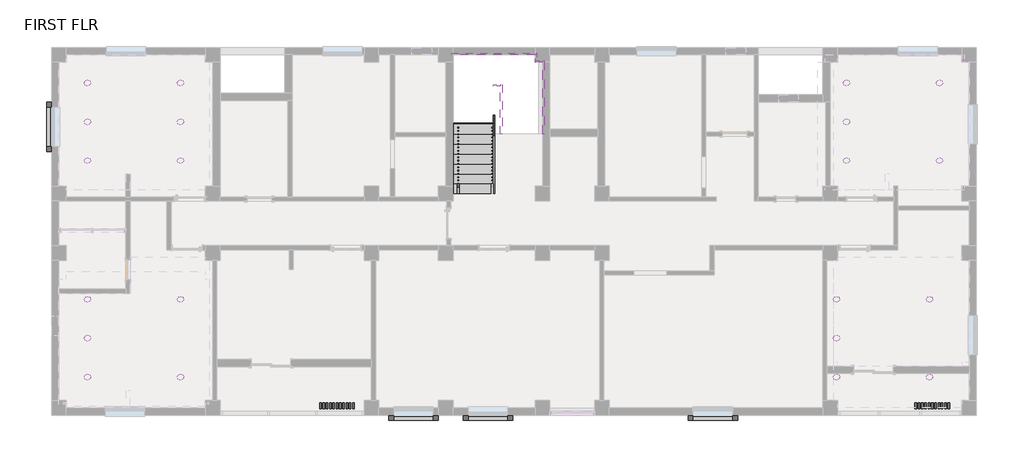
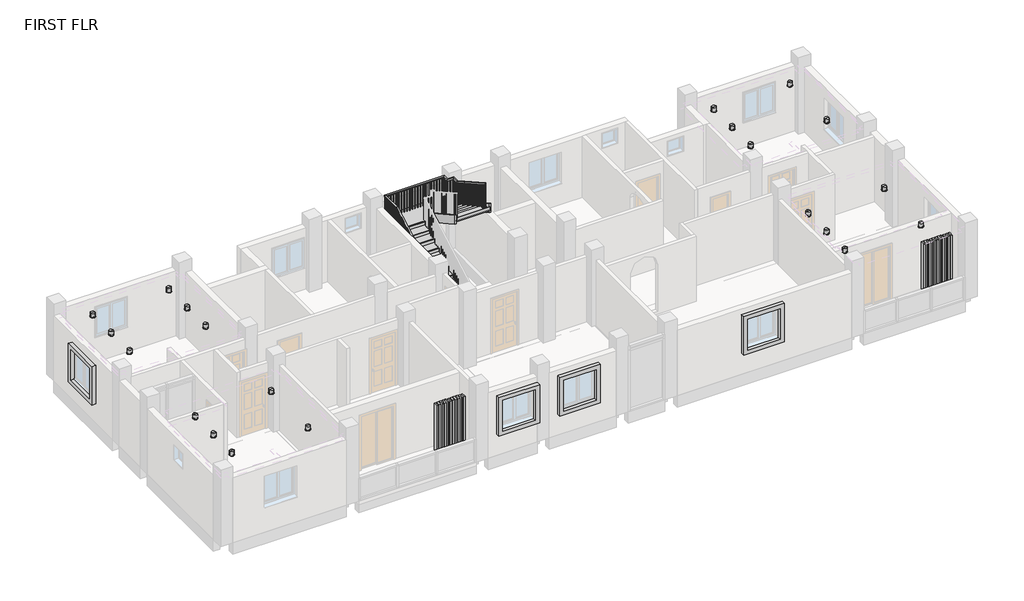
# One storey, part 5 of 5: 21 light fixtures, 8 members, 7 proxies, 1 railing, 1 stair flight.
"""IFC4 building model written with IfcOpenShell, lengths in millimetres."""

from ifc_helpers import new_model, si_unit, frame, origin, place, context, project, spatial, polyline, outline, extrude, faceted_brep, transform, mapped, element, save
from components import generic_models_14_generic_models_6_3cb9ea36, generic_models_17_generic_models_17_4194431e, generic_models_21_generic_models_21_07dc1754, light_modern_pendant_14774_baffle_cc9af11b, light_modern_pendant_14774_baffle_b3430626, stair_flight_d695bd93

model = new_model("IFC4")

# Units and contexts
model_context = context("Model", 3, world=origin())
ifc_project = project(units=[si_unit("LENGTHUNIT", "METRE", prefix="MILLI")], contexts=[model_context])

# Site, building, storey
site = spatial("IfcSite", under=ifc_project)
building = spatial("IfcBuilding", under=site)
storey = spatial("IfcBuildingStorey", under=building, Name="FIRST FLR", Elevation=3352.8)

# Proxies
placement = place(None, origin())
generic_models_14_generic_models_6_shape = generic_models_14_generic_models_6_3cb9ea36(model_context)
element("IfcBuildingElementProxy", 1, Name="Generic Models 14 : Generic Models 6", ObjectType="Generic Models 14 : Generic Models 6", at=placement, inside=storey, context=model_context, shape_type="MappedRepresentation", body=[
    mapped(generic_models_14_generic_models_6_shape, transform((18288.0, 190.5, -457.2), x_axis=(1.0, 0.0, 0.0), y_axis=(0.0, 1.0, 0.0), z_axis=(0.0, 0.0, 1.0))),
])
generic_models_17_generic_models_17_shape = generic_models_17_generic_models_17_4194431e(model_context)
element("IfcBuildingElementProxy", 2, Name="Generic Models 19 : Generic Models 17", ObjectType="Generic Models 19 : Generic Models 17", at=placement, inside=storey, context=model_context, shape_type="MappedRepresentation", body=[
    mapped(generic_models_17_generic_models_17_shape, transform((0.0, 0.0, -6096.0), x_axis=(1.0, 0.0, 0.0), y_axis=(0.0, 1.0, 0.0), z_axis=(0.0, 0.0, 1.0))),
])
generic_models_21_generic_models_21_shape = generic_models_21_generic_models_21_07dc1754(model_context)
element("IfcBuildingElementProxy", 3, Name="Generic Models 23 : Generic Models 21", ObjectType="Generic Models 23 : Generic Models 21", at=placement, inside=storey, context=model_context, shape_type="MappedRepresentation", body=[
    mapped(generic_models_21_generic_models_21_shape, transform((0.0, 0.0, -6096.0), x_axis=(1.0, 0.0, 0.0), y_axis=(0.0, 1.0, 0.0), z_axis=(0.0, 0.0, 1.0))),
])
element("IfcBuildingElementProxy", 4, Name="Generic Models 27 : Generic Models 21", ObjectType="Generic Models 27 : Generic Models 21", at=placement, inside=storey, context=model_context, shape_type="MappedRepresentation", body=[
    mapped(generic_models_21_generic_models_21_shape, transform((-6905.3372689, 0.0, -6096.0), x_axis=(1.0, 0.0, 0.0), y_axis=(0.0, 1.0, 0.0), z_axis=(0.0, 0.0, 1.0))),
])
element("IfcBuildingElementProxy", 5, Name="Generic Models 29 : Generic Models 21", ObjectType="Generic Models 29 : Generic Models 21", at=placement, inside=storey, context=model_context, shape_type="MappedRepresentation", body=[
    mapped(generic_models_21_generic_models_21_shape, transform((-6905.3372689, 0.0, -6096.0), x_axis=(1.0, 0.0, 0.0), y_axis=(0.0, 1.0, 0.0), z_axis=(0.0, 0.0, 1.0))),
])
element("IfcBuildingElementProxy", 6, Name="Generic Models 32 : Generic Models 21", ObjectType="Generic Models 32 : Generic Models 21", at=placement, inside=storey, context=model_context, shape_type="MappedRepresentation", body=[
    mapped(generic_models_21_generic_models_21_shape, transform((-9191.3372689, 0.0, -6096.0), x_axis=(1.0, 0.0, 0.0), y_axis=(0.0, 1.0, 0.0), z_axis=(0.0, 0.0, 1.0))),
])
element("IfcBuildingElementProxy", 7, Name="Generic Models 8 : Generic Models 6", ObjectType="Generic Models 8 : Generic Models 6", at=placement, inside=storey, context=model_context, shape_type="MappedRepresentation", body=[
    mapped(generic_models_14_generic_models_6_shape, transform((0.0, 190.5, -457.2), x_axis=(1.0, 0.0, 0.0), y_axis=(0.0, 1.0, 0.0), z_axis=(0.0, 0.0, 1.0))),
])

# Light fixtures
light_modern_pendant_14774_baffle_shape = light_modern_pendant_14774_baffle_cc9af11b(model_context)
element("IfcLightFixture", 8, ObjectType="LIGHT_-_MODERN_PENDANT_14774 : Baffle", at=placement, inside=storey, context=model_context, shape_type="MappedRepresentation", body=[
    mapped(light_modern_pendant_14774_baffle_shape, transform((-14269.0456086, -897.3794704, 3479.8), x_axis=(1.0, 0.0, 0.0), y_axis=(0.0, 1.0, 0.0), z_axis=(0.0, 0.0, 1.0))),
])
element("IfcLightFixture", 9, ObjectType="LIGHT_-_MODERN_PENDANT_14774 : Baffle", at=placement, inside=storey, context=model_context, shape_type="MappedRepresentation", body=[
    mapped(light_modern_pendant_14774_baffle_shape, transform((-14269.0456086, -3284.9794704, 3479.8), x_axis=(1.0, 0.0, 0.0), y_axis=(0.0, 1.0, 0.0), z_axis=(0.0, 0.0, 1.0))),
])
element("IfcLightFixture", 10, ObjectType="LIGHT_-_MODERN_PENDANT_14774 : Baffle", at=placement, inside=storey, context=model_context, shape_type="MappedRepresentation", body=[
    mapped(light_modern_pendant_14774_baffle_shape, transform((-14269.0456086, -2091.1794704, 3479.8), x_axis=(1.0, 0.0, 0.0), y_axis=(0.0, 1.0, 0.0), z_axis=(0.0, 0.0, 1.0))),
])
element("IfcLightFixture", 11, ObjectType="LIGHT_-_MODERN_PENDANT_14774 : Baffle", at=placement, inside=storey, context=model_context, shape_type="MappedRepresentation", body=[
    mapped(light_modern_pendant_14774_baffle_shape, transform((9048.1543914, -897.3794704, 3479.8), x_axis=(1.0, 0.0, 0.0), y_axis=(0.0, 1.0, 0.0), z_axis=(0.0, 0.0, 1.0))),
])
element("IfcLightFixture", 12, ObjectType="LIGHT_-_MODERN_PENDANT_14774 : Baffle", at=placement, inside=storey, context=model_context, shape_type="MappedRepresentation", body=[
    mapped(light_modern_pendant_14774_baffle_shape, transform((9048.1543914, -3284.9794704, 3479.8), x_axis=(1.0, 0.0, 0.0), y_axis=(0.0, 1.0, 0.0), z_axis=(0.0, 0.0, 1.0))),
])
element("IfcLightFixture", 13, ObjectType="LIGHT_-_MODERN_PENDANT_14774 : Baffle", at=placement, inside=storey, context=model_context, shape_type="MappedRepresentation", body=[
    mapped(light_modern_pendant_14774_baffle_shape, transform((9048.1543914, -2091.1794704, 3479.8), x_axis=(1.0, 0.0, 0.0), y_axis=(0.0, 1.0, 0.0), z_axis=(0.0, 0.0, 1.0))),
])
element("IfcLightFixture", 14, ObjectType="LIGHT_-_MODERN_PENDANT_14774 : Baffle", at=placement, inside=storey, context=model_context, shape_type="MappedRepresentation", body=[
    mapped(light_modern_pendant_14774_baffle_shape, transform((-14269.0456086, -7552.1794704, 3479.8), x_axis=(1.0, 0.0, 0.0), y_axis=(0.0, 1.0, 0.0), z_axis=(0.0, 0.0, 1.0))),
])
element("IfcLightFixture", 15, ObjectType="LIGHT_-_MODERN_PENDANT_14774 : Baffle", at=placement, inside=storey, context=model_context, shape_type="MappedRepresentation", body=[
    mapped(light_modern_pendant_14774_baffle_shape, transform((-14269.0456086, -9939.7794704, 3479.8), x_axis=(1.0, 0.0, 0.0), y_axis=(0.0, 1.0, 0.0), z_axis=(0.0, 0.0, 1.0))),
])
element("IfcLightFixture", 16, ObjectType="LIGHT_-_MODERN_PENDANT_14774 : Baffle", at=placement, inside=storey, context=model_context, shape_type="MappedRepresentation", body=[
    mapped(light_modern_pendant_14774_baffle_shape, transform((-14269.0456086, -8745.9794704, 3479.8), x_axis=(1.0, 0.0, 0.0), y_axis=(0.0, 1.0, 0.0), z_axis=(0.0, 0.0, 1.0))),
])
element("IfcLightFixture", 17, ObjectType="LIGHT_-_MODERN_PENDANT_14774 : Baffle", at=placement, inside=storey, context=model_context, shape_type="MappedRepresentation", body=[
    mapped(light_modern_pendant_14774_baffle_shape, transform((8743.3543914, -7552.1794704, 3479.8), x_axis=(1.0, 0.0, 0.0), y_axis=(0.0, 1.0, 0.0), z_axis=(0.0, 0.0, 1.0))),
])
element("IfcLightFixture", 18, ObjectType="LIGHT_-_MODERN_PENDANT_14774 : Baffle", at=placement, inside=storey, context=model_context, shape_type="MappedRepresentation", body=[
    mapped(light_modern_pendant_14774_baffle_shape, transform((8743.3543914, -9939.7794704, 3479.8), x_axis=(1.0, 0.0, 0.0), y_axis=(0.0, 1.0, 0.0), z_axis=(0.0, 0.0, 1.0))),
])
element("IfcLightFixture", 19, ObjectType="LIGHT_-_MODERN_PENDANT_14774 : Baffle", at=placement, inside=storey, context=model_context, shape_type="MappedRepresentation", body=[
    mapped(light_modern_pendant_14774_baffle_shape, transform((8743.3543914, -8745.9794704, 3479.8), x_axis=(1.0, 0.0, 0.0), y_axis=(0.0, 1.0, 0.0), z_axis=(0.0, 0.0, 1.0))),
])
light_modern_pendant_14774_baffle_2_shape = light_modern_pendant_14774_baffle_b3430626(model_context)
element("IfcLightFixture", 20, ObjectType="LIGHT_-_MODERN_PENDANT_14774 : Baffle", at=placement, inside=storey, context=model_context, shape_type="MappedRepresentation", body=[
    mapped(light_modern_pendant_14774_baffle_2_shape, transform((-11411.5456086, -897.3794704, 3479.8), x_axis=(-1.0, 0.0, 0.0), y_axis=(0.0, -1.0, 0.0), z_axis=(0.0, 0.0, 1.0))),
])
element("IfcLightFixture", 21, ObjectType="LIGHT_-_MODERN_PENDANT_14774 : Baffle", at=placement, inside=storey, context=model_context, shape_type="MappedRepresentation", body=[
    mapped(light_modern_pendant_14774_baffle_2_shape, transform((-11411.5456086, -3284.9794704, 3479.8), x_axis=(-1.0, 0.0, 0.0), y_axis=(0.0, -1.0, 0.0), z_axis=(0.0, 0.0, 1.0))),
])
element("IfcLightFixture", 22, ObjectType="LIGHT_-_MODERN_PENDANT_14774 : Baffle", at=placement, inside=storey, context=model_context, shape_type="MappedRepresentation", body=[
    mapped(light_modern_pendant_14774_baffle_2_shape, transform((-11411.5456086, -2091.1794704, 3479.8), x_axis=(-1.0, 0.0, 0.0), y_axis=(0.0, -1.0, 0.0), z_axis=(0.0, 0.0, 1.0))),
])
element("IfcLightFixture", 23, ObjectType="LIGHT_-_MODERN_PENDANT_14774 : Baffle", at=placement, inside=storey, context=model_context, shape_type="MappedRepresentation", body=[
    mapped(light_modern_pendant_14774_baffle_2_shape, transform((11905.6543914, -897.3794704, 3479.8), x_axis=(-1.0, 0.0, 0.0), y_axis=(0.0, -1.0, 0.0), z_axis=(0.0, 0.0, 1.0))),
])
element("IfcLightFixture", 24, ObjectType="LIGHT_-_MODERN_PENDANT_14774 : Baffle", at=placement, inside=storey, context=model_context, shape_type="MappedRepresentation", body=[
    mapped(light_modern_pendant_14774_baffle_2_shape, transform((11905.6543914, -3284.9794704, 3479.8), x_axis=(-1.0, 0.0, 0.0), y_axis=(0.0, -1.0, 0.0), z_axis=(0.0, 0.0, 1.0))),
])
element("IfcLightFixture", 25, ObjectType="LIGHT_-_MODERN_PENDANT_14774 : Baffle", at=placement, inside=storey, context=model_context, shape_type="MappedRepresentation", body=[
    mapped(light_modern_pendant_14774_baffle_2_shape, transform((-11411.5456086, -7552.1794704, 3479.8), x_axis=(-1.0, 0.0, 0.0), y_axis=(0.0, -1.0, 0.0), z_axis=(0.0, 0.0, 1.0))),
])
element("IfcLightFixture", 26, ObjectType="LIGHT_-_MODERN_PENDANT_14774 : Baffle", at=placement, inside=storey, context=model_context, shape_type="MappedRepresentation", body=[
    mapped(light_modern_pendant_14774_baffle_2_shape, transform((-11411.5456086, -9939.7794704, 3479.8), x_axis=(-1.0, 0.0, 0.0), y_axis=(0.0, -1.0, 0.0), z_axis=(0.0, 0.0, 1.0))),
])
element("IfcLightFixture", 27, ObjectType="LIGHT_-_MODERN_PENDANT_14774 : Baffle", at=placement, inside=storey, context=model_context, shape_type="MappedRepresentation", body=[
    mapped(light_modern_pendant_14774_baffle_2_shape, transform((11600.8543914, -7552.1794704, 3479.8), x_axis=(-1.0, 0.0, 0.0), y_axis=(0.0, -1.0, 0.0), z_axis=(0.0, 0.0, 1.0))),
])
element("IfcLightFixture", 28, ObjectType="LIGHT_-_MODERN_PENDANT_14774 : Baffle", at=placement, inside=storey, context=model_context, shape_type="MappedRepresentation", body=[
    mapped(light_modern_pendant_14774_baffle_2_shape, transform((11600.8543914, -9939.7794704, 3479.8), x_axis=(-1.0, 0.0, 0.0), y_axis=(0.0, -1.0, 0.0), z_axis=(0.0, 0.0, 1.0))),
])

# Members
element("IfcMember", 29, ObjectType="Stringer - 2\" Width", at=placement, inside=storey, context=model_context, shape_type="SweptSolid", body=[
    extrude(outline(polyline([(-4300.9794704, 3352.8), (-4300.9794704, 3560.3983948), (-879.896581, 5461.0), (-252.2749676, 5461.0), (-4047.0349676, 3352.8), (-4300.9794704, 3352.8)])), frame((-3080.3456086, 0.0, 0.0), z_axis=(1.0, 0.0, 0.0), x_axis=(0.0, 1.0, 0.0)), (0.0, 0.0, 1.0), 50.8),
])
element("IfcMember", 30, ObjectType="Stringer - 2\" Width", at=placement, inside=storey, context=model_context, shape_type="SweptSolid", body=[
    extrude(outline(polyline([(-3080.3456086, -33.7794704), (-3080.3456086, 17.0205296), (-467.6083398, 17.0205296), (-518.4083398, -33.7794704), (-3080.3456086, -33.7794704)])), frame((0.0, 0.0, 5156.2), z_axis=(0.0, 0.0, 1.0), x_axis=(1.0, 0.0, 0.0)), (0.0, 0.0, 1.0), 304.8),
])
element("IfcMember", 31, ObjectType="Stringer - 2\" Width", at=placement, inside=storey, context=model_context, shape_type="SweptSolid", body=[
    extrude(outline(polyline([(-518.4083398, -33.7794704), (-467.6083398, 17.0205296), (-467.6083398, -211.5794704), (-518.4083398, -262.3794704), (-518.4083398, -33.7794704)])), frame((0.0, 0.0, 5156.2), z_axis=(0.0, 0.0, 1.0), x_axis=(1.0, 0.0, 0.0)), (0.0, 0.0, 1.0), 304.8),
])
element("IfcMember", 32, ObjectType="Stringer - 2\" Width", at=placement, inside=storey, context=model_context, shape_type="SweptSolid", body=[
    extrude(outline(polyline([(-518.4083398, -262.3794704), (-467.6083398, -211.5794704), (-289.8083398, -211.5794704), (-289.8083398, -262.3794704), (-518.4083398, -262.3794704)])), frame((0.0, 0.0, 5156.2), z_axis=(0.0, 0.0, 1.0), x_axis=(1.0, 0.0, 0.0)), (0.0, 0.0, 1.0), 304.8),
])
element("IfcMember", 33, ObjectType="Stringer - 2\" Width", at=placement, inside=storey, context=model_context, shape_type="SweptSolid", body=[
    extrude(outline(polyline([(-211.5794704, 5183.1761726), (-211.5794704, 5156.2), (-790.6439732, 5156.2), (-2472.1794704, 6090.3863873), (-2472.1794704, 6439.0650614), (-211.5794704, 5183.1761726)])), frame((-289.8083398, 0.0, 0.0), z_axis=(1.0, 0.0, 0.0), x_axis=(0.0, 1.0, 0.0)), (0.0, 0.0, 1.0), 50.8),
])
element("IfcMember", 34, ObjectType="Stringer - 2\" Width", at=placement, inside=storey, context=model_context, shape_type="SweptSolid", body=[
    extrude(outline(polyline([(-4300.9794704, 3352.8), (-4300.9794704, 3560.3983948), (-998.9794704, 5394.8428392), (-998.9794704, 5046.1641651), (-4047.0349676, 3352.8), (-4300.9794704, 3352.8)])), frame((-1810.3456086, 0.0, 0.0), z_axis=(1.0, 0.0, 0.0), x_axis=(0.0, 1.0, 0.0)), (0.0, 0.0, 1.0), 50.8),
])
element("IfcMember", 35, ObjectType="Stringer - 2\" Width", at=placement, inside=storey, context=model_context, shape_type="SweptSolid", body=[
    extrude(outline(polyline([(-1810.3456086, -998.9794704), (-1810.3456086, -948.1794704), (-1585.2083398, -948.1794704), (-1585.2083398, -998.9794704), (-1810.3456086, -998.9794704)])), frame((0.0, 0.0, 5156.2), z_axis=(0.0, 0.0, 1.0), x_axis=(1.0, 0.0, 0.0)), (0.0, 0.0, 1.0), 304.8),
])
element("IfcMember", 36, ObjectType="Stringer - 2\" Width", at=placement, inside=storey, context=model_context, shape_type="SweptSolid", body=[
    extrude(outline(polyline([(-948.1794704, 5592.3983948), (-948.1794704, 5243.7197207), (-2472.1794704, 6090.3863873), (-2472.1794704, 6439.0650614), (-948.1794704, 5592.3983948)])), frame((-1585.2083398, 0.0, 0.0), z_axis=(1.0, 0.0, 0.0), x_axis=(0.0, 1.0, 0.0)), (0.0, 0.0, 1.0), 50.8),
])

# Railing
element("IfcRailing", 37, ObjectType="Handrail - Rectangular", at=placement, inside=storey, context=model_context, shape_type="SolidModel", body=[
    faceted_brep([(-2902.5456086, -4300.9794704, 4436.5333333), (-2902.5456086, -4300.9794704, 4378.420221), (-2851.7456086, -4300.9794704, 4378.420221), (-2851.7456086, -4300.9794704, 4436.5333333), (-2902.5456086, -948.1794704, 6299.2), (-2902.5456086, -935.0158682, 6248.4), (-2851.7456086, -935.0158682, 6248.4), (-2851.7456086, -948.1794704, 6299.2), (-2902.5456086, -160.7794704, 6299.2), (-2902.5456086, -160.7794704, 6248.4), (-2851.7456086, -211.5794704, 6248.4), (-2851.7456086, -211.5794704, 6299.2), (-645.4083398, -160.7794704, 6299.2), (-645.4083398, -160.7794704, 6248.4), (-696.2083398, -211.5794704, 6248.4), (-696.2083398, -211.5794704, 6299.2), (-645.4083398, -389.3794704, 6299.2), (-645.4083398, -389.3794704, 6248.4), (-696.2083398, -440.1794704, 6248.4), (-696.2083398, -440.1794704, 6299.2), (-416.8083398, -389.3794704, 6299.2), (-416.8083398, -389.3794704, 6248.4), (-467.6083398, -440.1794704, 6248.4), (-467.6083398, -440.1794704, 6299.2), (-416.8083398, -643.3794704, 6299.2), (-416.8083398, -656.5430727, 6248.4), (-467.6083398, -656.5430727, 6248.4), (-467.6083398, -643.3794704, 6299.2), (-416.8083398, -2472.1794704, 7315.2), (-467.6083398, -2472.1794704, 7315.2), (-467.6083398, -2472.1794704, 7257.0868876), (-416.8083398, -2472.1794704, 7257.0868876)], [[[0, 1, 2, 3]], [[1, 0, 4, 5]], [[2, 1, 5, 6]], [[3, 2, 6, 7]], [[0, 3, 7, 4]], [[5, 4, 8, 9]], [[6, 5, 9, 10]], [[7, 6, 10, 11]], [[4, 7, 11, 8]], [[9, 8, 12, 13]], [[10, 9, 13, 14]], [[11, 10, 14, 15]], [[8, 11, 15, 12]], [[13, 12, 16, 17]], [[14, 13, 17, 18]], [[15, 14, 18, 19]], [[12, 15, 19, 16]], [[17, 16, 20, 21]], [[18, 17, 21, 22]], [[19, 18, 22, 23]], [[16, 19, 23, 20]], [[21, 20, 24, 25]], [[22, 21, 25, 26]], [[23, 22, 26, 27]], [[20, 23, 27, 24]], [[28, 29, 30, 31]], [[25, 24, 28, 31]], [[26, 25, 31, 30]], [[27, 26, 30, 29]], [[24, 27, 29, 28]]]),
    extrude(outline(polyline([(-2437.2544704, 7237.6841099), (-2437.2544704, 6231.4666667), (-2456.3044704, 6231.4666667), (-2456.3044704, 7248.2674432), (-2437.2544704, 7237.6841099)])), frame((-451.7333398, 0.0, 0.0), z_axis=(1.0, 0.0, 0.0), x_axis=(0.0, 1.0, 0.0)), (0.0, 0.0, 1.0), 19.05),
    extrude(outline(polyline([(-2335.6544704, 7181.2396654), (-2335.6544704, 6231.4666667), (-2354.7044704, 6231.4666667), (-2354.7044704, 7191.8229988), (-2335.6544704, 7181.2396654)])), frame((-451.7333398, 0.0, 0.0), z_axis=(1.0, 0.0, 0.0), x_axis=(0.0, 1.0, 0.0)), (0.0, 0.0, 1.0), 19.05),
    extrude(outline(polyline([(-2234.0544704, 7124.795221), (-2234.0544704, 6231.4666667), (-2253.1044704, 6231.4666667), (-2253.1044704, 7135.3785543), (-2234.0544704, 7124.795221)])), frame((-451.7333398, 0.0, 0.0), z_axis=(1.0, 0.0, 0.0), x_axis=(0.0, 1.0, 0.0)), (0.0, 0.0, 1.0), 19.05),
    extrude(outline(polyline([(-2132.4544704, 7068.3507765), (-2132.4544704, 6062.1333333), (-2151.5044704, 6062.1333333), (-2151.5044704, 7078.9341099), (-2132.4544704, 7068.3507765)])), frame((-451.7333398, 0.0, 0.0), z_axis=(1.0, 0.0, 0.0), x_axis=(0.0, 1.0, 0.0)), (0.0, 0.0, 1.0), 19.05),
    extrude(outline(polyline([(-2030.8544704, 7011.9063321), (-2030.8544704, 6062.1333333), (-2049.9044704, 6062.1333333), (-2049.9044704, 7022.4896654), (-2030.8544704, 7011.9063321)])), frame((-451.7333398, 0.0, 0.0), z_axis=(1.0, 0.0, 0.0), x_axis=(0.0, 1.0, 0.0)), (0.0, 0.0, 1.0), 19.05),
    extrude(outline(polyline([(-1929.2544704, 6955.4618876), (-1929.2544704, 6062.1333333), (-1948.3044704, 6062.1333333), (-1948.3044704, 6966.045221), (-1929.2544704, 6955.4618876)])), frame((-451.7333398, 0.0, 0.0), z_axis=(1.0, 0.0, 0.0), x_axis=(0.0, 1.0, 0.0)), (0.0, 0.0, 1.0), 19.05),
    extrude(outline(polyline([(-1827.6544704, 6899.0174432), (-1827.6544704, 5892.8), (-1846.7044704, 5892.8), (-1846.7044704, 6909.6007765), (-1827.6544704, 6899.0174432)])), frame((-451.7333398, 0.0, 0.0), z_axis=(1.0, 0.0, 0.0), x_axis=(0.0, 1.0, 0.0)), (0.0, 0.0, 1.0), 19.05),
    extrude(outline(polyline([(-1726.0544704, 6842.5729988), (-1726.0544704, 5892.8), (-1745.1044704, 5892.8), (-1745.1044704, 6853.1563321), (-1726.0544704, 6842.5729988)])), frame((-451.7333398, 0.0, 0.0), z_axis=(1.0, 0.0, 0.0), x_axis=(0.0, 1.0, 0.0)), (0.0, 0.0, 1.0), 19.05),
    extrude(outline(polyline([(-1624.4544704, 6786.1285543), (-1624.4544704, 5892.8), (-1643.5044704, 5892.8), (-1643.5044704, 6796.7118876), (-1624.4544704, 6786.1285543)])), frame((-451.7333398, 0.0, 0.0), z_axis=(1.0, 0.0, 0.0), x_axis=(0.0, 1.0, 0.0)), (0.0, 0.0, 1.0), 19.05),
    extrude(outline(polyline([(-1522.8544704, 6729.6841099), (-1522.8544704, 5723.4666667), (-1541.9044704, 5723.4666667), (-1541.9044704, 6740.2674432), (-1522.8544704, 6729.6841099)])), frame((-451.7333398, 0.0, 0.0), z_axis=(1.0, 0.0, 0.0), x_axis=(0.0, 1.0, 0.0)), (0.0, 0.0, 1.0), 19.05),
    extrude(outline(polyline([(-1421.2544704, 6673.2396654), (-1421.2544704, 5723.4666667), (-1440.3044704, 5723.4666667), (-1440.3044704, 6683.8229988), (-1421.2544704, 6673.2396654)])), frame((-451.7333398, 0.0, 0.0), z_axis=(1.0, 0.0, 0.0), x_axis=(0.0, 1.0, 0.0)), (0.0, 0.0, 1.0), 19.05),
    extrude(outline(polyline([(-1319.6544704, 6616.795221), (-1319.6544704, 5723.4666667), (-1338.7044704, 5723.4666667), (-1338.7044704, 6627.3785543), (-1319.6544704, 6616.795221)])), frame((-451.7333398, 0.0, 0.0), z_axis=(1.0, 0.0, 0.0), x_axis=(0.0, 1.0, 0.0)), (0.0, 0.0, 1.0), 19.05),
    extrude(outline(polyline([(-1218.0544704, 6560.3507765), (-1218.0544704, 5554.1333333), (-1237.1044704, 5554.1333333), (-1237.1044704, 6570.9341099), (-1218.0544704, 6560.3507765)])), frame((-451.7333398, 0.0, 0.0), z_axis=(1.0, 0.0, 0.0), x_axis=(0.0, 1.0, 0.0)), (0.0, 0.0, 1.0), 19.05),
    extrude(outline(polyline([(-1116.4544704, 6503.9063321), (-1116.4544704, 5554.1333333), (-1135.5044704, 5554.1333333), (-1135.5044704, 6514.4896654), (-1116.4544704, 6503.9063321)])), frame((-451.7333398, 0.0, 0.0), z_axis=(1.0, 0.0, 0.0), x_axis=(0.0, 1.0, 0.0)), (0.0, 0.0, 1.0), 19.05),
    extrude(outline(polyline([(-1014.8544704, 6447.4618876), (-1014.8544704, 5554.1333333), (-1033.9044704, 5554.1333333), (-1033.9044704, 6458.045221), (-1014.8544704, 6447.4618876)])), frame((-451.7333398, 0.0, 0.0), z_axis=(1.0, 0.0, 0.0), x_axis=(0.0, 1.0, 0.0)), (0.0, 0.0, 1.0), 19.05),
    extrude(outline(polyline([(-913.2544704, 6391.0174432), (-913.2544704, 5384.8), (-932.3044704, 5384.8), (-932.3044704, 6401.6007765), (-913.2544704, 6391.0174432)])), frame((-451.7333398, 0.0, 0.0), z_axis=(1.0, 0.0, 0.0), x_axis=(0.0, 1.0, 0.0)), (0.0, 0.0, 1.0), 19.05),
    extrude(outline(polyline([(-811.6544704, 6334.5729988), (-811.6544704, 5384.8), (-830.7044704, 5384.8), (-830.7044704, 6345.1563321), (-811.6544704, 6334.5729988)])), frame((-451.7333398, 0.0, 0.0), z_axis=(1.0, 0.0, 0.0), x_axis=(0.0, 1.0, 0.0)), (0.0, 0.0, 1.0), 19.05),
    extrude(outline(polyline([(-710.0544704, 6278.1285543), (-710.0544704, 5384.8), (-729.1044704, 5384.8), (-729.1044704, 6288.7118876), (-710.0544704, 6278.1285543)])), frame((-451.7333398, 0.0, 0.0), z_axis=(1.0, 0.0, 0.0), x_axis=(0.0, 1.0, 0.0)), (0.0, 0.0, 1.0), 19.05),
    extrude(outline(polyline([(-432.6833398, -608.4544704), (-432.6833398, -627.5044704), (-451.7333398, -627.5044704), (-451.7333398, -608.4544704), (-432.6833398, -608.4544704)])), frame((0.0, 0.0, 5384.8), z_axis=(0.0, 0.0, 1.0), x_axis=(1.0, 0.0, 0.0)), (0.0, 0.0, 1.0), 863.6),
    extrude(outline(polyline([(-432.6833398, -506.8544704), (-432.6833398, -525.9044704), (-451.7333398, -525.9044704), (-451.7333398, -506.8544704), (-432.6833398, -506.8544704)])), frame((0.0, 0.0, 5384.8), z_axis=(0.0, 0.0, 1.0), x_axis=(1.0, 0.0, 0.0)), (0.0, 0.0, 1.0), 863.6),
    extrude(outline(polyline([(-477.1333398, -405.2544704), (-458.0833398, -405.2544704), (-458.0833398, -424.3044704), (-477.1333398, -424.3044704), (-477.1333398, -405.2544704)])), frame((0.0, 0.0, 5384.8), z_axis=(0.0, 0.0, 1.0), x_axis=(1.0, 0.0, 0.0)), (0.0, 0.0, 1.0), 863.6),
    extrude(outline(polyline([(-578.7333398, -405.2544704), (-559.6833398, -405.2544704), (-559.6833398, -424.3044704), (-578.7333398, -424.3044704), (-578.7333398, -405.2544704)])), frame((0.0, 0.0, 5384.8), z_axis=(0.0, 0.0, 1.0), x_axis=(1.0, 0.0, 0.0)), (0.0, 0.0, 1.0), 863.6),
    extrude(outline(polyline([(-661.2833398, -379.8544704), (-661.2833398, -398.9044704), (-680.3333398, -398.9044704), (-680.3333398, -379.8544704), (-661.2833398, -379.8544704)])), frame((0.0, 0.0, 5384.8), z_axis=(0.0, 0.0, 1.0), x_axis=(1.0, 0.0, 0.0)), (0.0, 0.0, 1.0), 863.6),
    extrude(outline(polyline([(-661.2833398, -278.2544704), (-661.2833398, -297.3044704), (-680.3333398, -297.3044704), (-680.3333398, -278.2544704), (-661.2833398, -278.2544704)])), frame((0.0, 0.0, 5384.8), z_axis=(0.0, 0.0, 1.0), x_axis=(1.0, 0.0, 0.0)), (0.0, 0.0, 1.0), 863.6),
    extrude(outline(polyline([(-753.0706086, -176.6544704), (-734.0206086, -176.6544704), (-734.0206086, -195.7044704), (-753.0706086, -195.7044704), (-753.0706086, -176.6544704)])), frame((0.0, 0.0, 5384.8), z_axis=(0.0, 0.0, 1.0), x_axis=(1.0, 0.0, 0.0)), (0.0, 0.0, 1.0), 863.6),
    extrude(outline(polyline([(-854.6706086, -176.6544704), (-835.6206086, -176.6544704), (-835.6206086, -195.7044704), (-854.6706086, -195.7044704), (-854.6706086, -176.6544704)])), frame((0.0, 0.0, 5384.8), z_axis=(0.0, 0.0, 1.0), x_axis=(1.0, 0.0, 0.0)), (0.0, 0.0, 1.0), 863.6),
    extrude(outline(polyline([(-956.2706086, -176.6544704), (-937.2206086, -176.6544704), (-937.2206086, -195.7044704), (-956.2706086, -195.7044704), (-956.2706086, -176.6544704)])), frame((0.0, 0.0, 5384.8), z_axis=(0.0, 0.0, 1.0), x_axis=(1.0, 0.0, 0.0)), (0.0, 0.0, 1.0), 863.6),
    extrude(outline(polyline([(-1057.8706086, -176.6544704), (-1038.8206086, -176.6544704), (-1038.8206086, -195.7044704), (-1057.8706086, -195.7044704), (-1057.8706086, -176.6544704)])), frame((0.0, 0.0, 5384.8), z_axis=(0.0, 0.0, 1.0), x_axis=(1.0, 0.0, 0.0)), (0.0, 0.0, 1.0), 863.6),
    extrude(outline(polyline([(-1159.4706086, -176.6544704), (-1140.4206086, -176.6544704), (-1140.4206086, -195.7044704), (-1159.4706086, -195.7044704), (-1159.4706086, -176.6544704)])), frame((0.0, 0.0, 5384.8), z_axis=(0.0, 0.0, 1.0), x_axis=(1.0, 0.0, 0.0)), (0.0, 0.0, 1.0), 863.6),
    extrude(outline(polyline([(-1261.0706086, -176.6544704), (-1242.0206086, -176.6544704), (-1242.0206086, -195.7044704), (-1261.0706086, -195.7044704), (-1261.0706086, -176.6544704)])), frame((0.0, 0.0, 5384.8), z_axis=(0.0, 0.0, 1.0), x_axis=(1.0, 0.0, 0.0)), (0.0, 0.0, 1.0), 863.6),
    extrude(outline(polyline([(-1362.6706086, -176.6544704), (-1343.6206086, -176.6544704), (-1343.6206086, -195.7044704), (-1362.6706086, -195.7044704), (-1362.6706086, -176.6544704)])), frame((0.0, 0.0, 5384.8), z_axis=(0.0, 0.0, 1.0), x_axis=(1.0, 0.0, 0.0)), (0.0, 0.0, 1.0), 863.6),
    extrude(outline(polyline([(-1464.2706086, -176.6544704), (-1445.2206086, -176.6544704), (-1445.2206086, -195.7044704), (-1464.2706086, -195.7044704), (-1464.2706086, -176.6544704)])), frame((0.0, 0.0, 5384.8), z_axis=(0.0, 0.0, 1.0), x_axis=(1.0, 0.0, 0.0)), (0.0, 0.0, 1.0), 863.6),
    extrude(outline(polyline([(-1565.8706086, -176.6544704), (-1546.8206086, -176.6544704), (-1546.8206086, -195.7044704), (-1565.8706086, -195.7044704), (-1565.8706086, -176.6544704)])), frame((0.0, 0.0, 5384.8), z_axis=(0.0, 0.0, 1.0), x_axis=(1.0, 0.0, 0.0)), (0.0, 0.0, 1.0), 863.6),
    extrude(outline(polyline([(-1667.4706086, -176.6544704), (-1648.4206086, -176.6544704), (-1648.4206086, -195.7044704), (-1667.4706086, -195.7044704), (-1667.4706086, -176.6544704)])), frame((0.0, 0.0, 5384.8), z_axis=(0.0, 0.0, 1.0), x_axis=(1.0, 0.0, 0.0)), (0.0, 0.0, 1.0), 863.6),
    extrude(outline(polyline([(-1769.0706086, -176.6544704), (-1750.0206086, -176.6544704), (-1750.0206086, -195.7044704), (-1769.0706086, -195.7044704), (-1769.0706086, -176.6544704)])), frame((0.0, 0.0, 5384.8), z_axis=(0.0, 0.0, 1.0), x_axis=(1.0, 0.0, 0.0)), (0.0, 0.0, 1.0), 863.6),
    extrude(outline(polyline([(-1870.6706086, -176.6544704), (-1851.6206086, -176.6544704), (-1851.6206086, -195.7044704), (-1870.6706086, -195.7044704), (-1870.6706086, -176.6544704)])), frame((0.0, 0.0, 5384.8), z_axis=(0.0, 0.0, 1.0), x_axis=(1.0, 0.0, 0.0)), (0.0, 0.0, 1.0), 863.6),
    extrude(outline(polyline([(-1972.2706086, -176.6544704), (-1953.2206086, -176.6544704), (-1953.2206086, -195.7044704), (-1972.2706086, -195.7044704), (-1972.2706086, -176.6544704)])), frame((0.0, 0.0, 5384.8), z_axis=(0.0, 0.0, 1.0), x_axis=(1.0, 0.0, 0.0)), (0.0, 0.0, 1.0), 863.6),
    extrude(outline(polyline([(-2073.8706086, -176.6544704), (-2054.8206086, -176.6544704), (-2054.8206086, -195.7044704), (-2073.8706086, -195.7044704), (-2073.8706086, -176.6544704)])), frame((0.0, 0.0, 5384.8), z_axis=(0.0, 0.0, 1.0), x_axis=(1.0, 0.0, 0.0)), (0.0, 0.0, 1.0), 863.6),
    extrude(outline(polyline([(-2175.4706086, -176.6544704), (-2156.4206086, -176.6544704), (-2156.4206086, -195.7044704), (-2175.4706086, -195.7044704), (-2175.4706086, -176.6544704)])), frame((0.0, 0.0, 5384.8), z_axis=(0.0, 0.0, 1.0), x_axis=(1.0, 0.0, 0.0)), (0.0, 0.0, 1.0), 863.6),
    extrude(outline(polyline([(-2277.0706086, -176.6544704), (-2258.0206086, -176.6544704), (-2258.0206086, -195.7044704), (-2277.0706086, -195.7044704), (-2277.0706086, -176.6544704)])), frame((0.0, 0.0, 5384.8), z_axis=(0.0, 0.0, 1.0), x_axis=(1.0, 0.0, 0.0)), (0.0, 0.0, 1.0), 863.6),
    extrude(outline(polyline([(-2378.6706086, -176.6544704), (-2359.6206086, -176.6544704), (-2359.6206086, -195.7044704), (-2378.6706086, -195.7044704), (-2378.6706086, -176.6544704)])), frame((0.0, 0.0, 5384.8), z_axis=(0.0, 0.0, 1.0), x_axis=(1.0, 0.0, 0.0)), (0.0, 0.0, 1.0), 863.6),
    extrude(outline(polyline([(-2480.2706086, -176.6544704), (-2461.2206086, -176.6544704), (-2461.2206086, -195.7044704), (-2480.2706086, -195.7044704), (-2480.2706086, -176.6544704)])), frame((0.0, 0.0, 5384.8), z_axis=(0.0, 0.0, 1.0), x_axis=(1.0, 0.0, 0.0)), (0.0, 0.0, 1.0), 863.6),
    extrude(outline(polyline([(-2581.8706086, -176.6544704), (-2562.8206086, -176.6544704), (-2562.8206086, -195.7044704), (-2581.8706086, -195.7044704), (-2581.8706086, -176.6544704)])), frame((0.0, 0.0, 5384.8), z_axis=(0.0, 0.0, 1.0), x_axis=(1.0, 0.0, 0.0)), (0.0, 0.0, 1.0), 863.6),
    extrude(outline(polyline([(-2683.4706086, -176.6544704), (-2664.4206086, -176.6544704), (-2664.4206086, -195.7044704), (-2683.4706086, -195.7044704), (-2683.4706086, -176.6544704)])), frame((0.0, 0.0, 5384.8), z_axis=(0.0, 0.0, 1.0), x_axis=(1.0, 0.0, 0.0)), (0.0, 0.0, 1.0), 863.6),
    extrude(outline(polyline([(-2785.0706086, -176.6544704), (-2766.0206086, -176.6544704), (-2766.0206086, -195.7044704), (-2785.0706086, -195.7044704), (-2785.0706086, -176.6544704)])), frame((0.0, 0.0, 5384.8), z_axis=(0.0, 0.0, 1.0), x_axis=(1.0, 0.0, 0.0)), (0.0, 0.0, 1.0), 863.6),
    extrude(outline(polyline([(-2886.6706086, -246.5044704), (-2886.6706086, -227.4544704), (-2867.6206086, -227.4544704), (-2867.6206086, -246.5044704), (-2886.6706086, -246.5044704)])), frame((0.0, 0.0, 5384.8), z_axis=(0.0, 0.0, 1.0), x_axis=(1.0, 0.0, 0.0)), (0.0, 0.0, 1.0), 863.6),
    extrude(outline(polyline([(-2886.6706086, -348.1044704), (-2886.6706086, -329.0544704), (-2867.6206086, -329.0544704), (-2867.6206086, -348.1044704), (-2886.6706086, -348.1044704)])), frame((0.0, 0.0, 5384.8), z_axis=(0.0, 0.0, 1.0), x_axis=(1.0, 0.0, 0.0)), (0.0, 0.0, 1.0), 863.6),
    extrude(outline(polyline([(-2886.6706086, -449.7044704), (-2886.6706086, -430.6544704), (-2867.6206086, -430.6544704), (-2867.6206086, -449.7044704), (-2886.6706086, -449.7044704)])), frame((0.0, 0.0, 5384.8), z_axis=(0.0, 0.0, 1.0), x_axis=(1.0, 0.0, 0.0)), (0.0, 0.0, 1.0), 863.6),
    extrude(outline(polyline([(-2886.6706086, -551.3044704), (-2886.6706086, -532.2544704), (-2867.6206086, -532.2544704), (-2867.6206086, -551.3044704), (-2886.6706086, -551.3044704)])), frame((0.0, 0.0, 5384.8), z_axis=(0.0, 0.0, 1.0), x_axis=(1.0, 0.0, 0.0)), (0.0, 0.0, 1.0), 863.6),
    extrude(outline(polyline([(-2886.6706086, -652.9044704), (-2886.6706086, -633.8544704), (-2867.6206086, -633.8544704), (-2867.6206086, -652.9044704), (-2886.6706086, -652.9044704)])), frame((0.0, 0.0, 5384.8), z_axis=(0.0, 0.0, 1.0), x_axis=(1.0, 0.0, 0.0)), (0.0, 0.0, 1.0), 863.6),
    extrude(outline(polyline([(-2886.6706086, -754.5044704), (-2886.6706086, -735.4544704), (-2867.6206086, -735.4544704), (-2867.6206086, -754.5044704), (-2886.6706086, -754.5044704)])), frame((0.0, 0.0, 5384.8), z_axis=(0.0, 0.0, 1.0), x_axis=(1.0, 0.0, 0.0)), (0.0, 0.0, 1.0), 863.6),
    extrude(outline(polyline([(-2886.6706086, -856.1044704), (-2886.6706086, -837.0544704), (-2867.6206086, -837.0544704), (-2867.6206086, -856.1044704), (-2886.6706086, -856.1044704)])), frame((0.0, 0.0, 5384.8), z_axis=(0.0, 0.0, 1.0), x_axis=(1.0, 0.0, 0.0)), (0.0, 0.0, 1.0), 863.6),
    extrude(outline(polyline([(-938.6544704, 6246.3785543), (-938.6544704, 5384.8), (-957.7044704, 5384.8), (-957.7044704, 6235.795221), (-938.6544704, 6246.3785543)])), frame((-2886.6706086, 0.0, 0.0), z_axis=(1.0, 0.0, 0.0), x_axis=(0.0, 1.0, 0.0)), (0.0, 0.0, 1.0), 19.05),
    extrude(outline(polyline([(-1040.2544704, 6189.9341099), (-1040.2544704, 5215.4666667), (-1059.3044704, 5215.4666667), (-1059.3044704, 6179.3507765), (-1040.2544704, 6189.9341099)])), frame((-2886.6706086, 0.0, 0.0), z_axis=(1.0, 0.0, 0.0), x_axis=(0.0, 1.0, 0.0)), (0.0, 0.0, 1.0), 19.05),
    extrude(outline(polyline([(-1141.8544704, 6133.4896654), (-1141.8544704, 5215.4666667), (-1160.9044704, 5215.4666667), (-1160.9044704, 6122.9063321), (-1141.8544704, 6133.4896654)])), frame((-2886.6706086, 0.0, 0.0), z_axis=(1.0, 0.0, 0.0), x_axis=(0.0, 1.0, 0.0)), (0.0, 0.0, 1.0), 19.05),
    extrude(outline(polyline([(-1243.4544704, 6077.045221), (-1243.4544704, 5215.4666667), (-1262.5044704, 5215.4666667), (-1262.5044704, 6066.4618876), (-1243.4544704, 6077.045221)])), frame((-2886.6706086, 0.0, 0.0), z_axis=(1.0, 0.0, 0.0), x_axis=(0.0, 1.0, 0.0)), (0.0, 0.0, 1.0), 19.05),
    extrude(outline(polyline([(-1345.0544704, 6020.6007765), (-1345.0544704, 5046.1333333), (-1364.1044704, 5046.1333333), (-1364.1044704, 6010.0174432), (-1345.0544704, 6020.6007765)])), frame((-2886.6706086, 0.0, 0.0), z_axis=(1.0, 0.0, 0.0), x_axis=(0.0, 1.0, 0.0)), (0.0, 0.0, 1.0), 19.05),
    extrude(outline(polyline([(-1446.6544704, 5964.1563321), (-1446.6544704, 5046.1333333), (-1465.7044704, 5046.1333333), (-1465.7044704, 5953.5729988), (-1446.6544704, 5964.1563321)])), frame((-2886.6706086, 0.0, 0.0), z_axis=(1.0, 0.0, 0.0), x_axis=(0.0, 1.0, 0.0)), (0.0, 0.0, 1.0), 19.05),
    extrude(outline(polyline([(-1548.2544704, 5907.7118876), (-1548.2544704, 5046.1333333), (-1567.3044704, 5046.1333333), (-1567.3044704, 5897.1285543), (-1548.2544704, 5907.7118876)])), frame((-2886.6706086, 0.0, 0.0), z_axis=(1.0, 0.0, 0.0), x_axis=(0.0, 1.0, 0.0)), (0.0, 0.0, 1.0), 19.05),
    extrude(outline(polyline([(-1649.8544704, 5851.2674432), (-1649.8544704, 4876.8), (-1668.9044704, 4876.8), (-1668.9044704, 5840.6841099), (-1649.8544704, 5851.2674432)])), frame((-2886.6706086, 0.0, 0.0), z_axis=(1.0, 0.0, 0.0), x_axis=(0.0, 1.0, 0.0)), (0.0, 0.0, 1.0), 19.05),
    extrude(outline(polyline([(-1751.4544704, 5794.8229988), (-1751.4544704, 4876.8), (-1770.5044704, 4876.8), (-1770.5044704, 5784.2396654), (-1751.4544704, 5794.8229988)])), frame((-2886.6706086, 0.0, 0.0), z_axis=(1.0, 0.0, 0.0), x_axis=(0.0, 1.0, 0.0)), (0.0, 0.0, 1.0), 19.05),
    extrude(outline(polyline([(-1853.0544704, 5738.3785543), (-1853.0544704, 4876.8), (-1872.1044704, 4876.8), (-1872.1044704, 5727.795221), (-1853.0544704, 5738.3785543)])), frame((-2886.6706086, 0.0, 0.0), z_axis=(1.0, 0.0, 0.0), x_axis=(0.0, 1.0, 0.0)), (0.0, 0.0, 1.0), 19.05),
    extrude(outline(polyline([(-1954.6544704, 5681.9341099), (-1954.6544704, 4707.4666667), (-1973.7044704, 4707.4666667), (-1973.7044704, 5671.3507765), (-1954.6544704, 5681.9341099)])), frame((-2886.6706086, 0.0, 0.0), z_axis=(1.0, 0.0, 0.0), x_axis=(0.0, 1.0, 0.0)), (0.0, 0.0, 1.0), 19.05),
    extrude(outline(polyline([(-2056.2544704, 5625.4896654), (-2056.2544704, 4707.4666667), (-2075.3044704, 4707.4666667), (-2075.3044704, 5614.9063321), (-2056.2544704, 5625.4896654)])), frame((-2886.6706086, 0.0, 0.0), z_axis=(1.0, 0.0, 0.0), x_axis=(0.0, 1.0, 0.0)), (0.0, 0.0, 1.0), 19.05),
    extrude(outline(polyline([(-2157.8544704, 5569.045221), (-2157.8544704, 4707.4666667), (-2176.9044704, 4707.4666667), (-2176.9044704, 5558.4618876), (-2157.8544704, 5569.045221)])), frame((-2886.6706086, 0.0, 0.0), z_axis=(1.0, 0.0, 0.0), x_axis=(0.0, 1.0, 0.0)), (0.0, 0.0, 1.0), 19.05),
    extrude(outline(polyline([(-2259.4544704, 5512.6007765), (-2259.4544704, 4538.1333333), (-2278.5044704, 4538.1333333), (-2278.5044704, 5502.0174432), (-2259.4544704, 5512.6007765)])), frame((-2886.6706086, 0.0, 0.0), z_axis=(1.0, 0.0, 0.0), x_axis=(0.0, 1.0, 0.0)), (0.0, 0.0, 1.0), 19.05),
    extrude(outline(polyline([(-2361.0544704, 5456.1563321), (-2361.0544704, 4538.1333333), (-2380.1044704, 4538.1333333), (-2380.1044704, 5445.5729988), (-2361.0544704, 5456.1563321)])), frame((-2886.6706086, 0.0, 0.0), z_axis=(1.0, 0.0, 0.0), x_axis=(0.0, 1.0, 0.0)), (0.0, 0.0, 1.0), 19.05),
    extrude(outline(polyline([(-2462.6544704, 5399.7118876), (-2462.6544704, 4538.1333333), (-2481.7044704, 4538.1333333), (-2481.7044704, 5389.1285543), (-2462.6544704, 5399.7118876)])), frame((-2886.6706086, 0.0, 0.0), z_axis=(1.0, 0.0, 0.0), x_axis=(0.0, 1.0, 0.0)), (0.0, 0.0, 1.0), 19.05),
    extrude(outline(polyline([(-2564.2544704, 5343.2674432), (-2564.2544704, 4368.8), (-2583.3044704, 4368.8), (-2583.3044704, 5332.6841099), (-2564.2544704, 5343.2674432)])), frame((-2886.6706086, 0.0, 0.0), z_axis=(1.0, 0.0, 0.0), x_axis=(0.0, 1.0, 0.0)), (0.0, 0.0, 1.0), 19.05),
    extrude(outline(polyline([(-2665.8544704, 5286.8229988), (-2665.8544704, 4368.8), (-2684.9044704, 4368.8), (-2684.9044704, 5276.2396654), (-2665.8544704, 5286.8229988)])), frame((-2886.6706086, 0.0, 0.0), z_axis=(1.0, 0.0, 0.0), x_axis=(0.0, 1.0, 0.0)), (0.0, 0.0, 1.0), 19.05),
    extrude(outline(polyline([(-2767.4544704, 5230.3785543), (-2767.4544704, 4368.8), (-2786.5044704, 4368.8), (-2786.5044704, 5219.795221), (-2767.4544704, 5230.3785543)])), frame((-2886.6706086, 0.0, 0.0), z_axis=(1.0, 0.0, 0.0), x_axis=(0.0, 1.0, 0.0)), (0.0, 0.0, 1.0), 19.05),
    extrude(outline(polyline([(-2869.0544704, 5173.9341099), (-2869.0544704, 4199.4666667), (-2888.1044704, 4199.4666667), (-2888.1044704, 5163.3507765), (-2869.0544704, 5173.9341099)])), frame((-2886.6706086, 0.0, 0.0), z_axis=(1.0, 0.0, 0.0), x_axis=(0.0, 1.0, 0.0)), (0.0, 0.0, 1.0), 19.05),
    extrude(outline(polyline([(-2970.6544704, 5117.4896654), (-2970.6544704, 4199.4666667), (-2989.7044704, 4199.4666667), (-2989.7044704, 5106.9063321), (-2970.6544704, 5117.4896654)])), frame((-2886.6706086, 0.0, 0.0), z_axis=(1.0, 0.0, 0.0), x_axis=(0.0, 1.0, 0.0)), (0.0, 0.0, 1.0), 19.05),
    extrude(outline(polyline([(-3072.2544704, 5061.045221), (-3072.2544704, 4199.4666667), (-3091.3044704, 4199.4666667), (-3091.3044704, 5050.4618876), (-3072.2544704, 5061.045221)])), frame((-2886.6706086, 0.0, 0.0), z_axis=(1.0, 0.0, 0.0), x_axis=(0.0, 1.0, 0.0)), (0.0, 0.0, 1.0), 19.05),
    extrude(outline(polyline([(-3173.8544704, 5004.6007765), (-3173.8544704, 4030.1333333), (-3192.9044704, 4030.1333333), (-3192.9044704, 4994.0174432), (-3173.8544704, 5004.6007765)])), frame((-2886.6706086, 0.0, 0.0), z_axis=(1.0, 0.0, 0.0), x_axis=(0.0, 1.0, 0.0)), (0.0, 0.0, 1.0), 19.05),
    extrude(outline(polyline([(-3275.4544704, 4948.1563321), (-3275.4544704, 4030.1333333), (-3294.5044704, 4030.1333333), (-3294.5044704, 4937.5729988), (-3275.4544704, 4948.1563321)])), frame((-2886.6706086, 0.0, 0.0), z_axis=(1.0, 0.0, 0.0), x_axis=(0.0, 1.0, 0.0)), (0.0, 0.0, 1.0), 19.05),
    extrude(outline(polyline([(-3377.0544704, 4891.7118876), (-3377.0544704, 4030.1333333), (-3396.1044704, 4030.1333333), (-3396.1044704, 4881.1285543), (-3377.0544704, 4891.7118876)])), frame((-2886.6706086, 0.0, 0.0), z_axis=(1.0, 0.0, 0.0), x_axis=(0.0, 1.0, 0.0)), (0.0, 0.0, 1.0), 19.05),
    extrude(outline(polyline([(-3478.6544704, 4835.2674432), (-3478.6544704, 3860.8), (-3497.7044704, 3860.8), (-3497.7044704, 4824.6841099), (-3478.6544704, 4835.2674432)])), frame((-2886.6706086, 0.0, 0.0), z_axis=(1.0, 0.0, 0.0), x_axis=(0.0, 1.0, 0.0)), (0.0, 0.0, 1.0), 19.05),
    extrude(outline(polyline([(-3580.2544704, 4778.8229988), (-3580.2544704, 3860.8), (-3599.3044704, 3860.8), (-3599.3044704, 4768.2396654), (-3580.2544704, 4778.8229988)])), frame((-2886.6706086, 0.0, 0.0), z_axis=(1.0, 0.0, 0.0), x_axis=(0.0, 1.0, 0.0)), (0.0, 0.0, 1.0), 19.05),
    extrude(outline(polyline([(-3681.8544704, 4722.3785543), (-3681.8544704, 3860.8), (-3700.9044704, 3860.8), (-3700.9044704, 4711.795221), (-3681.8544704, 4722.3785543)])), frame((-2886.6706086, 0.0, 0.0), z_axis=(1.0, 0.0, 0.0), x_axis=(0.0, 1.0, 0.0)), (0.0, 0.0, 1.0), 19.05),
    extrude(outline(polyline([(-3783.4544704, 4665.9341099), (-3783.4544704, 3691.4666667), (-3802.5044704, 3691.4666667), (-3802.5044704, 4655.3507765), (-3783.4544704, 4665.9341099)])), frame((-2886.6706086, 0.0, 0.0), z_axis=(1.0, 0.0, 0.0), x_axis=(0.0, 1.0, 0.0)), (0.0, 0.0, 1.0), 19.05),
    extrude(outline(polyline([(-3885.0544704, 4609.4896654), (-3885.0544704, 3691.4666667), (-3904.1044704, 3691.4666667), (-3904.1044704, 4598.9063321), (-3885.0544704, 4609.4896654)])), frame((-2886.6706086, 0.0, 0.0), z_axis=(1.0, 0.0, 0.0), x_axis=(0.0, 1.0, 0.0)), (0.0, 0.0, 1.0), 19.05),
    extrude(outline(polyline([(-3986.6544704, 4553.045221), (-3986.6544704, 3691.4666667), (-4005.7044704, 3691.4666667), (-4005.7044704, 4542.4618876), (-3986.6544704, 4553.045221)])), frame((-2886.6706086, 0.0, 0.0), z_axis=(1.0, 0.0, 0.0), x_axis=(0.0, 1.0, 0.0)), (0.0, 0.0, 1.0), 19.05),
    extrude(outline(polyline([(-4088.2544704, 4496.6007765), (-4088.2544704, 3522.1333333), (-4107.3044704, 3522.1333333), (-4107.3044704, 4486.0174432), (-4088.2544704, 4496.6007765)])), frame((-2886.6706086, 0.0, 0.0), z_axis=(1.0, 0.0, 0.0), x_axis=(0.0, 1.0, 0.0)), (0.0, 0.0, 1.0), 19.05),
    extrude(outline(polyline([(-4189.8544704, 4440.1563321), (-4189.8544704, 3522.1333333), (-4208.9044704, 3522.1333333), (-4208.9044704, 4429.5729988), (-4189.8544704, 4440.1563321)])), frame((-2886.6706086, 0.0, 0.0), z_axis=(1.0, 0.0, 0.0), x_axis=(0.0, 1.0, 0.0)), (0.0, 0.0, 1.0), 19.05),
    extrude(outline(polyline([(-451.7333398, -405.2544704), (-432.6833398, -405.2544704), (-432.6833398, -424.3044704), (-451.7333398, -424.3044704), (-451.7333398, -405.2544704)])), frame((0.0, 0.0, 5384.8), z_axis=(0.0, 0.0, 1.0), x_axis=(1.0, 0.0, 0.0)), (0.0, 0.0, 1.0), 863.6),
    extrude(outline(polyline([(-661.2833398, -405.2544704), (-661.2833398, -424.3044704), (-680.3333398, -424.3044704), (-680.3333398, -405.2544704), (-661.2833398, -405.2544704)])), frame((0.0, 0.0, 5384.8), z_axis=(0.0, 0.0, 1.0), x_axis=(1.0, 0.0, 0.0)), (0.0, 0.0, 1.0), 863.6),
    extrude(outline(polyline([(-680.3333398, -176.6544704), (-661.2833398, -176.6544704), (-661.2833398, -195.7044704), (-680.3333398, -195.7044704), (-680.3333398, -176.6544704)])), frame((0.0, 0.0, 5384.8), z_axis=(0.0, 0.0, 1.0), x_axis=(1.0, 0.0, 0.0)), (0.0, 0.0, 1.0), 863.6),
    extrude(outline(polyline([(-2886.6706086, -195.7044704), (-2886.6706086, -176.6544704), (-2867.6206086, -176.6544704), (-2867.6206086, -195.7044704), (-2886.6706086, -195.7044704)])), frame((0.0, 0.0, 5384.8), z_axis=(0.0, 0.0, 1.0), x_axis=(1.0, 0.0, 0.0)), (0.0, 0.0, 1.0), 863.6),
    extrude(outline(polyline([(-2453.1294704, 7246.5035543), (-2453.1294704, 6231.4666667), (-2472.1794704, 6231.4666667), (-2472.1794704, 7257.0868876), (-2453.1294704, 7246.5035543)])), frame((-451.7333398, 0.0, 0.0), z_axis=(1.0, 0.0, 0.0), x_axis=(0.0, 1.0, 0.0)), (0.0, 0.0, 1.0), 19.05),
    extrude(outline(polyline([(-4281.9294704, 4389.0035543), (-4281.9294704, 3522.1333333), (-4300.9794704, 3522.1333333), (-4300.9794704, 4378.420221), (-4281.9294704, 4389.0035543)])), frame((-2886.6706086, 0.0, 0.0), z_axis=(1.0, 0.0, 0.0), x_axis=(0.0, 1.0, 0.0)), (0.0, 0.0, 1.0), 19.05),
])

# Stair flight
stair_flight_shape = stair_flight_d695bd93(model_context)
element("IfcStairFlight", 38, ObjectType="2\" Tread 1\" Nosing 1/4\" Riser", at=placement, inside=storey, context=model_context, shape_type="MappedRepresentation", body=[
    mapped(stair_flight_shape, transform((0.0, 0.0, 0.0), x_axis=(1.0, 0.0, 0.0), y_axis=(0.0, 1.0, 0.0), z_axis=(0.0, 0.0, 1.0))),
])

save(model, "model.ifc")

# Revit data of these elements
# Type "LIGHT_-_MODERN_PENDANT_14774 : Baffle"
#   Assembly Code = "D5020220"
#   Lamp = "A-19"
#   Wattage Comments = "60"
#   Wattage = 7.27067 W
#   built-in parameter 1150110 = 1 (stored number, unit not read)
#   built-in parameter 1114217 = 1 (stored number, unit not read)
#   Tilt Angle = 60.00°
#   built-in parameter 1150109 = 1 (stored number, unit not read)
#   built-in parameter 1150113 = 1 (stored number, unit not read)
#   built-in parameter 1010507 = 1.5708 (stored number, unit not read)
#   built-in parameter 1010506 = 0.523599 (stored number, unit not read)
#   built-in parameter 1150105 = 3611.05 (stored number, unit not read)
#   built-in parameter 1150115 = 1 (stored number, unit not read)
#   Light Source Symbol Length = 10' - 0"
#   built-in parameter 1150112 = 1 (stored number, unit not read)
#   built-in parameter 1150114 = 1 (stored number, unit not read)
#   built-in parameter 1150107 = 3200 (stored number, unit not read)
#   built-in parameter 1150106 = 36.1105 (stored number, unit not read)
#   built-in parameter 1150104 = 13.8 (stored number, unit not read)
#   built-in parameter 1114218 = 1 (stored number, unit not read)
#   built-in parameter 1150133 = 10 (stored number, unit not read)
#   Depth = 0' - 8"
#   Diameter = 0' - 6"
#   Lumens = 1080 lm
#   Wall Washer = no
#   Wall Wash Trim = no
#   built-in parameter 1150134 = 3
#   Reflector Cone = no
#   built-in parameter 1150132 = 2
#   Fresnel Lens = no
#   Color Filter = 16777215
#   Baffle = yes
#   Wall Wash Reflector [instance default] = none
#   Reflector [instance default] = none
#   Light Trim = Metal - Paint Finish - Ivory,Glossy
#   Fresnel Material [instance default] = none
#   Dimming Lamp Color Temperature Shift = (empty or 0)
#   Default Elevation = 0
# Type "Handrail - Rectangular"
#   Assembly Code = "C2010400"
#   built-in parameter 1008612 = 0.0416667 (stored number, unit not read)
#   built-in parameter 1008611 = 0.0416667 (stored number, unit not read)
#   built-in parameter 1008609 = 0.333333 (stored number, unit not read)
#   built-in parameter 1008604 = 0.166667 (stored number, unit not read)
#   built-in parameter 1008603 = 0.166667 (stored number, unit not read)
#   Railing Height = 3' - 0"
#   built-in parameter 1008630 = 2
#   built-in parameter 1008610 = 2
#   built-in parameter 1008618 = Baluster - Square : 3/4"
# Element 1 (IfcBuildingElementProxy, "Generic Models 14 : Generic Models 6")
#   Phase Created = New Construction
#   Materials on its faces: "TEAK BROWN COLOUR"
# Element 2 (IfcBuildingElementProxy, "Generic Models 19 : Generic Models 17")
#   Phase Created = New Construction
#   Materials on its faces: "TEAK BROWN COLOUR"
# Element 3 (IfcBuildingElementProxy, "Generic Models 23 : Generic Models 21")
#   Phase Created = New Construction
#   Materials on its faces: "TEAK BROWN COLOUR"
# Element 4 (IfcBuildingElementProxy, "Generic Models 27 : Generic Models 21")
#   Phase Created = New Construction
#   Materials on its faces: "TEAK BROWN COLOUR"
# Element 5 (IfcBuildingElementProxy, "Generic Models 29 : Generic Models 21")
#   Phase Created = New Construction
#   Materials on its faces: "TEAK BROWN COLOUR"
# Element 6 (IfcBuildingElementProxy, "Generic Models 32 : Generic Models 21")
#   Phase Created = New Construction
#   Materials on its faces: "TEAK BROWN COLOUR"
# Element 7 (IfcBuildingElementProxy, "Generic Models 8 : Generic Models 6")
#   Phase Created = New Construction
#   Materials on its faces: "TEAK BROWN COLOUR"
# Element 8 (IfcLightFixture, "LIGHT_-_MODERN_PENDANT_14774 : Baffle")
#   Mark = "15"
#   Wall Wash Reflector = none
#   Reflector = none
#   Fresnel Material = none
#   Phase Created = New Construction
#   Materials on its faces: "Metal - Paint Finish - Ivory,Glossy"
# Element 9 (IfcLightFixture, "LIGHT_-_MODERN_PENDANT_14774 : Baffle")
#   Mark = "16"
#   Wall Wash Reflector = none
#   Reflector = none
#   Fresnel Material = none
#   Phase Created = New Construction
#   Materials on its faces: "Metal - Paint Finish - Ivory,Glossy"
# Element 10 (IfcLightFixture, "LIGHT_-_MODERN_PENDANT_14774 : Baffle")
#   Mark = "17"
#   Wall Wash Reflector = none
#   Reflector = none
#   Fresnel Material = none
#   Phase Created = New Construction
#   Materials on its faces: "Metal - Paint Finish - Ivory,Glossy"
# Element 11 (IfcLightFixture, "LIGHT_-_MODERN_PENDANT_14774 : Baffle")
#   Mark = "21"
#   Wall Wash Reflector = none
#   Reflector = none
#   Fresnel Material = none
#   Phase Created = New Construction
#   Materials on its faces: "Metal - Paint Finish - Ivory,Glossy"
# Element 12 (IfcLightFixture, "LIGHT_-_MODERN_PENDANT_14774 : Baffle")
#   Mark = "22"
#   Wall Wash Reflector = none
#   Reflector = none
#   Fresnel Material = none
#   Phase Created = New Construction
#   Materials on its faces: "Metal - Paint Finish - Ivory,Glossy"
# Element 13 (IfcLightFixture, "LIGHT_-_MODERN_PENDANT_14774 : Baffle")
#   Mark = "23"
#   Wall Wash Reflector = none
#   Reflector = none
#   Fresnel Material = none
#   Phase Created = New Construction
#   Materials on its faces: "Metal - Paint Finish - Ivory,Glossy"
# Element 14 (IfcLightFixture, "LIGHT_-_MODERN_PENDANT_14774 : Baffle")
#   Mark = "27"
#   Wall Wash Reflector = none
#   Reflector = none
#   Fresnel Material = none
#   Phase Created = New Construction
#   Materials on its faces: "Metal - Paint Finish - Ivory,Glossy"
# Element 15 (IfcLightFixture, "LIGHT_-_MODERN_PENDANT_14774 : Baffle")
#   Mark = "28"
#   Wall Wash Reflector = none
#   Reflector = none
#   Fresnel Material = none
#   Phase Created = New Construction
#   Materials on its faces: "Metal - Paint Finish - Ivory,Glossy"
# Element 16 (IfcLightFixture, "LIGHT_-_MODERN_PENDANT_14774 : Baffle")
#   Mark = "29"
#   Wall Wash Reflector = none
#   Reflector = none
#   Fresnel Material = none
#   Phase Created = New Construction
#   Materials on its faces: "Metal - Paint Finish - Ivory,Glossy"
# Element 17 (IfcLightFixture, "LIGHT_-_MODERN_PENDANT_14774 : Baffle")
#   Mark = "33"
#   Wall Wash Reflector = none
#   Reflector = none
#   Fresnel Material = none
#   Phase Created = New Construction
#   Materials on its faces: "Metal - Paint Finish - Ivory,Glossy"
# Element 18 (IfcLightFixture, "LIGHT_-_MODERN_PENDANT_14774 : Baffle")
#   Mark = "34"
#   Wall Wash Reflector = none
#   Reflector = none
#   Fresnel Material = none
#   Phase Created = New Construction
#   Materials on its faces: "Metal - Paint Finish - Ivory,Glossy"
# Element 19 (IfcLightFixture, "LIGHT_-_MODERN_PENDANT_14774 : Baffle")
#   Mark = "35"
#   Wall Wash Reflector = none
#   Reflector = none
#   Fresnel Material = none
#   Phase Created = New Construction
#   Materials on its faces: "Metal - Paint Finish - Ivory,Glossy"
# Element 20 (IfcLightFixture, "LIGHT_-_MODERN_PENDANT_14774 : Baffle")
#   Mark = "18"
#   Wall Wash Reflector = none
#   Reflector = none
#   Fresnel Material = none
#   Phase Created = New Construction
#   Materials on its faces: "Metal - Paint Finish - Ivory,Glossy"
# Element 21 (IfcLightFixture, "LIGHT_-_MODERN_PENDANT_14774 : Baffle")
#   Mark = "19"
#   Wall Wash Reflector = none
#   Reflector = none
#   Fresnel Material = none
#   Phase Created = New Construction
#   Materials on its faces: "Metal - Paint Finish - Ivory,Glossy"
# Element 22 (IfcLightFixture, "LIGHT_-_MODERN_PENDANT_14774 : Baffle")
#   Mark = "20"
#   Wall Wash Reflector = none
#   Reflector = none
#   Fresnel Material = none
#   Phase Created = New Construction
#   Materials on its faces: "Metal - Paint Finish - Ivory,Glossy"
# Element 23 (IfcLightFixture, "LIGHT_-_MODERN_PENDANT_14774 : Baffle")
#   Mark = "24"
#   Wall Wash Reflector = none
#   Reflector = none
#   Fresnel Material = none
#   Phase Created = New Construction
#   Materials on its faces: "Metal - Paint Finish - Ivory,Glossy"
# Element 24 (IfcLightFixture, "LIGHT_-_MODERN_PENDANT_14774 : Baffle")
#   Mark = "25"
#   Wall Wash Reflector = none
#   Reflector = none
#   Fresnel Material = none
#   Phase Created = New Construction
#   Materials on its faces: "Metal - Paint Finish - Ivory,Glossy"
# Element 25 (IfcLightFixture, "LIGHT_-_MODERN_PENDANT_14774 : Baffle")
#   Mark = "30"
#   Wall Wash Reflector = none
#   Reflector = none
#   Fresnel Material = none
#   Phase Created = New Construction
#   Materials on its faces: "Metal - Paint Finish - Ivory,Glossy"
# Element 26 (IfcLightFixture, "LIGHT_-_MODERN_PENDANT_14774 : Baffle")
#   Mark = "31"
#   Wall Wash Reflector = none
#   Reflector = none
#   Fresnel Material = none
#   Phase Created = New Construction
#   Materials on its faces: "Metal - Paint Finish - Ivory,Glossy"
# Element 27 (IfcLightFixture, "LIGHT_-_MODERN_PENDANT_14774 : Baffle")
#   Mark = "36"
#   Wall Wash Reflector = none
#   Reflector = none
#   Fresnel Material = none
#   Phase Created = New Construction
#   Materials on its faces: "Metal - Paint Finish - Ivory,Glossy"
# Element 28 (IfcLightFixture, "LIGHT_-_MODERN_PENDANT_14774 : Baffle")
#   Mark = "37"
#   Wall Wash Reflector = none
#   Reflector = none
#   Fresnel Material = none
#   Phase Created = New Construction
#   Materials on its faces: "Metal - Paint Finish - Ivory,Glossy"
# Elements 29, 30, 31, 32, 33, 34, 35, 36 (IfcMember, "Stringer - 2\" Width")
#   Phase Created = New Construction
# Element 37 (IfcRailing, "Handrail - Rectangular")
#   Phase Created = New Construction
# Element 38 (IfcStairFlight, "2\" Tread 1\" Nosing 1/4\" Riser")
#   Phase Created = New Construction
# Materials
#   "Metal - Paint Finish - Ivory,Glossy": colour RGB 247 247 239, transparency 0
#   "TEAK BROWN COLOUR": class "Generic", colour RGB 120 120 120, transparency 0, Cost = 0
